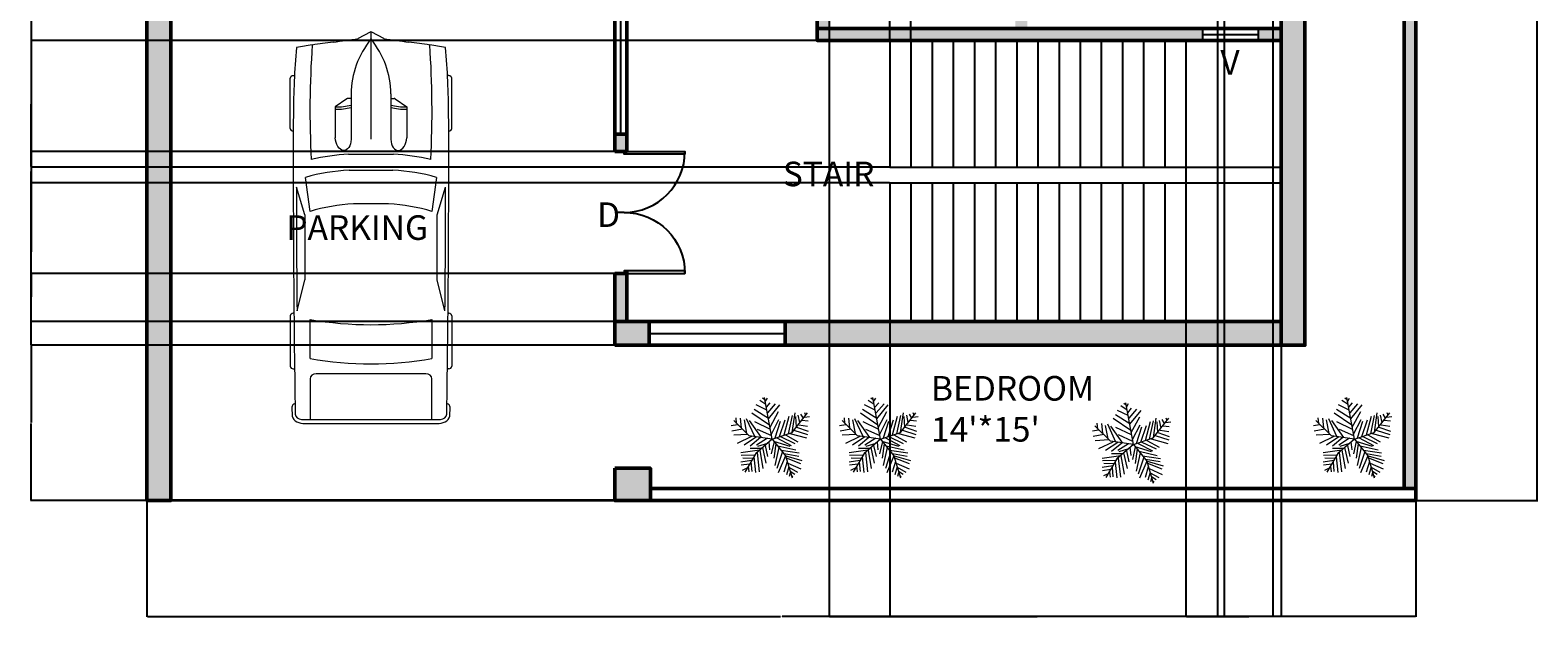
# Model space of a CAD drawing. Units: inches. Extents: x 2024 to 2594, y 643 to 1604.
# Tile 1 of 4: x 2024 to 2594, y 643 to 865. Entities that reach past the tile are written whole.
import ezdxf

# ---------------------------------------------------------------- set-up
doc = ezdxf.new("R2010")
doc.units = ezdxf.units.IN
for name, color, linetype, lineweight in [('A-ANNO-DIMS', 2, 'Continuous', 18), ('A-ANNO-TEXT', 7, 'Continuous', 18), ('A-AREA-IDEN', 7, 'Continuous', 25), ('A-FLOR-STRS', 7, 'Continuous', 25), ('A-WALL-PATT', 50, 'Continuous', 13), ('C-PRKG-VEHI', 8, 'Continuous', 18), ('C-PROP', 7, 'Continuous', 35), ('DOOR', 240, 'Continuous', 25), ('TREE', 102, 'Continuous', 18), ('WALL', 50, 'Continuous', 50), ('WIN', 140, 'Continuous', 25)]:
    doc.layers.add(name, color=color, linetype=linetype, lineweight=lineweight)
doc.styles.get("Standard").update_dxf_attribs({"font": 'arial.ttf'})
doc.dimstyles.get("Standard").update_dxf_attribs({"dimtxt": 0.18, "dimasz": 0.18, "dimexe": 0.18, "dimexo": 0.0625, "dimgap": 0.09, "dimtad": 0, "dimtih": 1, "dimtoh": 1, "dimdec": 4, "dimzin": 0, "dimdsep": 46, "dimtxsty": 'Standard', "dimcen": 0.09, "dimadec": 0, "dimazin": 0, "dimtfac": 1, "dimtdec": 4, "dimtofl": 0, "dimtmove": 0, "dimatfit": 3, "dimfxl": 1, "dimtolj": 1, "dimtzin": 0, "dimarcsym": 0})

# ---------------------------------------------------------------- blocks, each defined once
blk = doc.blocks.new('*U8')
for p, q in [((21.1, 37.41), (21.1, 36.83)), ((46.55, 38.89), (22.35, 38.89)), ((47.8, 37.39), (47.8, 37.41)), ((135.45, 37.07), (135.45, 37.41)), ((136.7, 38.89), (160.9, 38.89)), ((162.15, 37.41), (162.15, 36.77)), ((70.03, 31.54), (86.41, 29.35)), ((87.99, 31.87), (74.76, 35.92)), ((134.31, 35.6), (119.29, 31.78)), ((138.42, 29.35), (157.25, 29.35)), ((186.47, 29.35), (167.01, 29.35)), ((186.47, -33.5), (186.47, 33.5)), ((188.4, -32.76), (188.4, 32.76)), ((164.52, 26.39), (164.52, -26.39)), ((32.27, 11.63), (36.13, 17.17)), ((36.13, 17.17), (50.94, 17.17)), ((29.77, 9.51), (51.68, 9.51)), ((32.12, 9.51), (32.12, 11.15)), ((58.92, -10.77), (58.92, 10.77)), ((66.55, -10.53), (66.55, 10.53)), ((82.74, 8.5), (82.74, -8.5)), ((186.47, -10.53), (186.47, 10.53)), ((3.27, 6.13), (0.1, 0.41)), ((0, 0), (51.68, 0)), ((0.1, -0.41), (3.27, -6.13)), ((29.77, -9.51), (51.68, -9.51)), ((32.12, -9.51), (32.12, -11.15)), ((32.27, -11.63), (36.13, -17.17)), ((36.13, -17.17), (50.94, -17.17)), ((86.41, -29.35), (70.03, -31.54)), ((87.99, -31.87), (74.76, -35.92)), ((134.31, -35.6), (119.29, -31.78)), ((157.25, -29.35), (138.42, -29.35)), ((167.01, -29.35), (186.47, -29.35)), ((21.1, -37.41), (21.1, -36.83)), ((46.55, -38.89), (22.35, -38.89)), ((47.8, -37.39), (47.8, -37.41)), ((135.45, -37.07), (135.45, -37.41)), ((136.7, -38.89), (160.9, -38.89)), ((162.15, -37.41), (162.15, -36.77))]:
    blk.add_line(p, q)
for centre, major_axis, ratio, start_param, end_param in [((41.19, -490.86), (0, 528.23), 0.842304, 0.00281, 0.075598), ((22.35, 37.41), (0, -1.48), 0.842304, 3.141593, 4.712389), ((64.48, -10555.62), (0, 10593.03), 0.842304, -0.013397, 0.002797), ((46.55, 37.41), (0, 1.48), 0.842304, -1.570796, 0), ((136.7, 37.41), (0, -1.48), 0.842304, 3.141593, 4.712389), ((160.9, 37.41), (0, 1.48), 0.842304, -1.570796, 0), ((180.63, 35.84), (0, 2.22), 0.842304, -0.013017, 1.249894), ((64.48, -10556.36), (0, 10595.31), 0.842304, -0.013397, -0.013017), ((183.98, 33.5), (0, -2.96), 0.842304, 1.570796, 3.128196), ((183.98, 32.76), (0, -5.25), 0.842304, 1.570796, 3.128196), ((266.03, -27.52), (0, 313.31), 0.842304, 1.367076, 1.39176), ((37.47, -593.96), (0, -623.33), 0.842304, 3.096046, 3.200911), ((135.29, 5.39), (0, 81.77), 0.842304, 1.245306, 1.50788), ((64.48, -10555.62), (0, -10591.55), 0.842304, 3.133765, 3.140441), ((149.6, 2.8), (0, -79.58), 0.842304, 4.372215, 4.640744), ((95.79, -3666.35), (0, -3698.24), 0.842304, 3.134049, 3.144098), ((17.08, 0), (0, 147.02), 0.842304, 4.511394, 4.913384), ((35.91, 0), (0, 147.02), 0.842304, 4.511394, 4.913384), ((167.01, 26.39), (0, 2.96), 0.842304, 0, 1.570796), ((259.18, -27.52), (0, -305.3), 0.842304, 4.528606, 4.561838), ((134.4, 5.39), (0, -89.78), 0.842304, 4.449482, 4.652344), ((-204.49, 52.4), (0, -250.96), 0.842304, 1.385369, 1.434372), ((13.04, 17.01), (0, 27.42), 0.842304, 4.435146, 4.718221), ((14.2, 17.01), (0, 27.42), 0.842304, 4.435146, 4.718221), ((50.79, 13.34), (6.34, -0.36), 0.603834, -1.395552, 1.581315), ((29.77, -46.66), (0, 56.17), 0.842304, 0, 0.590319), ((32.75, 11.15), (0, 0.74), 0.842304, 0.879714, 1.570796), ((0.62, 0), (0, -0.74), 0.842304, 4.131459, 5.293319), ((-204.49, -52.4), (0, 250.96), 0.842304, -1.434372, -1.385369), ((29.77, 46.66), (0, 56.17), 0.842304, 2.551274, 3.141593), ((32.75, -11.15), (0, -0.74), 0.842304, 4.712389, 5.403472), ((13.04, -17.01), (0, -27.42), 0.842304, 1.564964, 1.848039), ((14.2, -17.01), (0, -27.42), 0.842304, 1.564964, 1.848039), ((134.4, -5.39), (0, -89.78), 0.842304, -1.510751, -1.307889), ((135.29, -5.39), (0, -81.77), 0.842304, -1.50788, -1.245306), ((149.6, -2.8), (0, -79.58), 0.842304, -1.499151, -1.230623), ((259.18, 27.52), (0, 305.3), 0.842304, 1.721348, 1.754579), ((266.03, 27.52), (0, 313.31), 0.842304, 1.749832, 1.774517), ((37.47, 593.96), (0, -623.33), 0.842304, -0.059319, 0.045547), ((167.01, -26.39), (0, -2.96), 0.842304, 4.712389, 6.283185), ((41.19, 490.86), (0, -528.23), 0.842304, -0.075598, -0.00281), ((64.48, 10555.62), (0, -10591.55), 0.842304, 0.001152, 0.007828), ((95.79, 3666.35), (0, -3698.24), 0.842304, -0.002505, 0.007544), ((183.98, -33.5), (0, 2.96), 0.842304, 3.15499, 4.712389), ((183.98, -32.76), (0, -5.25), 0.842304, 0.013397, 1.570796), ((22.35, -37.41), (0, 1.48), 0.842304, 1.570796, 3.141593), ((64.48, 10555.62), (0, 10593.03), 0.842304, 3.138796, 3.15499), ((46.55, -37.41), (0, -1.48), 0.842304, 0, 1.570796), ((136.7, -37.41), (0, -1.48), 0.842304, -1.570796, 0), ((160.9, -37.41), (0, 1.48), 0.842304, 3.141593, 4.712389), ((180.63, -35.84), (0, -2.22), 0.842304, -1.249894, 0.013017), ((64.48, 10556.36), (0, 10595.31), 0.842304, 3.15461, 3.15499)]:
    blk.add_ellipse(centre, major_axis=major_axis, ratio=ratio, start_param=start_param, end_param=end_param)
at = {"extrusion": (0, 0, -1)}
blk.add_ellipse((50.79, -13.34), major_axis=(6.34, 0.36), ratio=0.603834, start_param=-1.395552, end_param=1.581315, dxfattribs=at)
blk = doc.blocks.new('*U2')
for p, q in [((0, 0), (0, -6)), ((40, 0), (40, -6))]:
    blk.add_line(p, q)
blk.add_lwpolyline([(0, 0), (0, 40), (1.75, 40), (1.75, 0)], close=True)
blk.add_arc((0, 0), 40, 0, 90)
blk = doc.blocks.new('*U6')
for p, q in [((-7.288, 39.707), (-21.778, 46.673)), ((-8.737, 47.138), (-17.069, 52.711)), ((-10.186, 53.64), (-13.084, 55.962)), ((0, 0), (-10.5, 57)), ((-9.099, 51.782), (-6.563, 55.962)), ((-7.65, 43.423), (-2.578, 49.46)), ((-5.839, 35.992), (4.667, 48.067)), ((-5.114, 27.632), (10.463, 46.673)), ((-31.5, 4.5), (-52.5, 25.5)), ((-48.585, 21.131), (-49.309, 29.026)), ((-43.513, 28.561), (-42.427, 15.558)), ((-38.442, 26.239), (-34.819, 7.663)), ((-35.544, 28.097), (-24.314, 3.947)), ((-14.533, 2.09), (-30.834, 25.31)), ((-3.665, 19.273), (-27.574, 35.527)), ((-5.114, 28.097), (-24.676, 40.636)), ((-24.314, 23.917), (-2.941, 13.7)), ((-2.941, 16.486), (8.652, 37.85)), ((-1.129, 6.734), (9.014, 26.704)), ((3.942, 1.625), (11.187, 24.381)), ((10.101, 3.483), (17.708, 26.239)), ((16.259, 5.805), (23.142, 31.348)), ((22.055, 7.198), (27.489, 32.277)), ((27, 9), (48, 36)), ((27.127, 9.056), (31.112, 35.992)), ((31.836, 30.883), (32.561, 16.486)), ((35.096, 32.741), (37.27, 22.524)), ((38.719, 34.134), (41.979, 28.561)), ((40.53, 25.775), (48.862, 24.846)), ((43.791, 29.954), (51.036, 30.883)), ((44.153, 36.456), (45.239, 32.741)), ((-47.498, 19.737), (-55.83, 18.344)), ((-40.615, 13.7), (-55.105, 10.913)), ((-33.37, 6.269), (-52.207, 5.34)), ((-28.299, 3.483), (-47.86, -5.805)), ((-21.416, 3.018), (-38.079, -8.128)), ((0, 0), (-31.5, 4.5)), ((-15.982, 2.09), (-30.11, -9.521)), ((0, 0), (-22.5, -19.5)), ((-6.563, 1.161), (-21.416, -8.128)), ((-20.691, 13.7), (-1.129, 4.876)), ((0, 0), (27, 9)), ((0, 0), (18, -22.5)), ((6.478, 1.625), (26.04, -8.592)), ((11.187, 3.483), (30.749, -5.805)), ((18.07, 5.805), (35.096, -3.483)), ((24.229, 7.663), (46.688, 1.625)), ((29.662, 12.307), (48.137, 6.269)), ((33.285, 16.486), (48.862, 10.913)), ((36.183, 19.737), (48.137, 17.88)), ((-17.431, -15.094), (-42.789, -18.809)), ((-22.5, -19.5), (-37.5, -45)), ((-15.257, -12.772), (-30.11, -12.772)), ((-20.691, -18.345), (-17.793, -44.352)), ((-6.563, -5.805), (-19.967, -9.985)), ((-17.069, -15.094), (-12.721, -40.172)), ((-13.446, -11.378), (-8.737, -32.741)), ((-9.461, -8.592), (-6.201, -23.453)), ((-4.752, -3.483), (-3.665, -14.629)), ((2.493, -3.019), (-1.491, -20.202)), ((1.769, -2.555), (24.229, -9.521)), ((5.029, -6.27), (2.131, -25.775)), ((9.014, -11.378), (3.58, -35.992)), ((14.085, -16.951), (6.478, -40.172)), ((7.565, -9.056), (32.198, -14.629)), ((12.274, -15.094), (36.907, -18.809)), ((16.259, -19.738), (36.183, -22.989)), ((-28.299, -29.026), (-42.789, -31.348)), ((-24.314, -21.596), (-42.427, -22.06)), ((-30.834, -34.135), (-42.427, -35.528)), ((-34.457, -39.708), (-40.978, -42.494)), ((-26.849, -26.24), (-40.253, -25.775)), ((-32.646, -36.921), (-31.921, -44.352)), ((-29.023, -30.884), (-27.936, -43.887)), ((-25.038, -23.918), (-22.865, -45.281)), ((18.07, -22.524), (8.289, -45.745)), ((20.244, -30.419), (15.897, -44.816)), ((18, -22.5), (27, -52.5)), ((18.433, -22.524), (40.53, -29.026)), ((19.157, -25.311), (38.719, -33.206)), ((22.78, -37.85), (19.519, -48.532)), ((21.331, -32.741), (39.081, -40.636)), ((22.78, -38.314), (34.372, -44.816)), ((24.591, -45.745), (23.142, -50.854)), ((24.591, -43.423), (30.749, -47.603)), ((26.764, -49.925), (28.213, -50.854))]:
    blk.add_line(p, q)
blk = doc.blocks.new('*D25')
at = {"layer": 'A-ANNO-DIMS', "color": 0, "lineweight": -2, "transparency": 16777216}
for p, q in [((2068.27, 686.87), (2068.27, 642.95)), ((2548.27, 686.87), (2548.27, 642.95)), ((2068.45, 643.13), (2307.98, 643.13)), ((2548.09, 643.13), (2308.56, 643.13))]:
    blk.add_line(p, q, dxfattribs=at)
at = {"layer": 'A-ANNO-DIMS', "color": 0, "lineweight": 100, "transparency": 16777216}
for points in [[(2068.45, 643.16), (2068.45, 643.1), (2068.27, 643.13)], [(2548.09, 643.16), (2548.09, 643.1), (2548.27, 643.13)]]:
    blk.add_solid(points, dxfattribs=at)
at = {"layer": 'Defpoints', "color": 0, "lineweight": 100, "transparency": 16777216}
for p in [(2068.27, 686.93), (2548.27, 686.93), (2548.27, 643.13)]:
    blk.add_point(p, dxfattribs=at)
at = {"layer": 'A-ANNO-DIMS', "color": 0, "transparency": 16777216, "insert": (2308.27, 643.13), "char_height": 0.18, "attachment_point": 5}
blk.add_mtext('\\A1;480', dxfattribs=at)
blk = doc.blocks.new('*D26')
at = {"layer": 'A-ANNO-DIMS', "color": 0, "lineweight": -2, "transparency": 16777216}
for p, q in [((2548.34, 1526.93), (2594.37, 1526.93)), ((2594.19, 1526.75), (2594.19, 1107.11)), ((2594.19, 687.11), (2594.19, 1106.75)), ((2548.34, 686.93), (2594.37, 686.93))]:
    blk.add_line(p, q, dxfattribs=at)
at = {"layer": 'A-ANNO-DIMS', "color": 0, "lineweight": 100, "transparency": 16777216}
for points in [[(2594.16, 1526.75), (2594.22, 1526.75), (2594.19, 1526.93)], [(2594.16, 687.11), (2594.22, 687.11), (2594.19, 686.93)]]:
    blk.add_solid(points, dxfattribs=at)
at = {"layer": 'Defpoints', "color": 0, "lineweight": 100, "transparency": 16777216}
for p in [(2548.27, 1526.93), (2594.19, 1526.93), (2548.27, 686.93)]:
    blk.add_point(p, dxfattribs=at)
at = {"layer": 'A-ANNO-DIMS', "color": 0, "transparency": 16777216, "insert": (2594.19, 1106.93), "char_height": 0.18, "attachment_point": 5}
blk.add_mtext('\\A1;840', dxfattribs=at)
blk = doc.blocks.new('*D31')
at = {"layer": 'A-ANNO-DIMS', "color": 0, "lineweight": -2, "transparency": 16777216}
for p, q in [((2245.21, 745.67), (2024.29, 745.67)), ((2024.47, 745.49), (2024.47, 716.48)), ((2024.47, 687.11), (2024.47, 716.12)), ((2068.21, 686.93), (2024.29, 686.93))]:
    blk.add_line(p, q, dxfattribs=at)
at = {"layer": 'A-ANNO-DIMS', "color": 0, "lineweight": 100, "transparency": 16777216}
for points in [[(2024.44, 745.49), (2024.5, 745.49), (2024.47, 745.67)], [(2024.44, 687.11), (2024.5, 687.11), (2024.47, 686.93)]]:
    blk.add_solid(points, dxfattribs=at)
at = {"layer": 'Defpoints', "color": 0, "lineweight": 100, "transparency": 16777216}
for p in [(2024.47, 745.67), (2245.27, 745.67), (2068.27, 686.93)]:
    blk.add_point(p, dxfattribs=at)
at = {"layer": 'A-ANNO-DIMS', "color": 0, "transparency": 16777216, "insert": (2024.47, 716.3), "char_height": 0.18, "attachment_point": 5}
blk.add_mtext('\\A1;58.74', dxfattribs=at)
blk = doc.blocks.new('*D32')
at = {"layer": 'A-ANNO-DIMS', "color": 0, "lineweight": -2, "transparency": 16777216}
for p, q in [((2077.21, 877.43), (2024.29, 877.43)), ((2024.47, 877.25), (2024.47, 811.73)), ((2024.47, 745.85), (2024.47, 811.37)), ((2245.21, 745.67), (2024.29, 745.67))]:
    blk.add_line(p, q, dxfattribs=at)
at = {"layer": 'A-ANNO-DIMS', "color": 0, "lineweight": 100, "transparency": 16777216}
for points in [[(2024.44, 877.25), (2024.5, 877.25), (2024.47, 877.43)], [(2024.44, 745.85), (2024.5, 745.85), (2024.47, 745.67)]]:
    blk.add_solid(points, dxfattribs=at)
at = {"layer": 'Defpoints', "color": 0, "lineweight": 100, "transparency": 16777216}
for p in [(2024.47, 877.43), (2077.27, 877.43), (2245.27, 745.67)]:
    blk.add_point(p, dxfattribs=at)
at = {"layer": 'A-ANNO-DIMS', "color": 0, "transparency": 16777216, "insert": (2024.47, 811.55), "char_height": 0.18, "attachment_point": 5}
blk.add_mtext('\\A1;131.76', dxfattribs=at)
blk = doc.blocks.new('*D40')
at = {"layer": 'A-ANNO-DIMS', "color": 0, "lineweight": -2, "transparency": 16777216}
for p, q in [((2326.27, 1114.37), (2326.27, 642.95)), ((2473.27, 1114.37), (2473.27, 642.95)), ((2326.45, 643.13), (2399.49, 643.13)), ((2473.09, 643.13), (2400.05, 643.13))]:
    blk.add_line(p, q, dxfattribs=at)
at = {"layer": 'A-ANNO-DIMS', "color": 0, "lineweight": 100, "transparency": 16777216}
for points in [[(2326.45, 643.16), (2326.45, 643.1), (2326.27, 643.13)], [(2473.09, 643.16), (2473.09, 643.1), (2473.27, 643.13)]]:
    blk.add_solid(points, dxfattribs=at)
at = {"layer": 'Defpoints', "color": 0, "lineweight": 100, "transparency": 16777216}
for p in [(2326.27, 1114.43), (2473.27, 1114.43), (2473.27, 643.13)]:
    blk.add_point(p, dxfattribs=at)
at = {"layer": 'A-ANNO-DIMS', "color": 0, "transparency": 16777216, "insert": (2399.77, 643.13), "char_height": 0.18, "attachment_point": 5}
blk.add_mtext('\\A1;147', dxfattribs=at)
blk = doc.blocks.new('*D41')
at = {"layer": 'A-ANNO-DIMS', "color": 0, "lineweight": -2, "transparency": 16777216}
for p, q in [((2473.27, 1114.37), (2473.27, 642.95)), ((2497.27, 1090.37), (2497.27, 642.95)), ((2473.45, 643.13), (2485.05, 643.13)), ((2497.09, 643.13), (2485.49, 643.13))]:
    blk.add_line(p, q, dxfattribs=at)
at = {"layer": 'A-ANNO-DIMS', "color": 0, "lineweight": 100, "transparency": 16777216}
for points in [[(2473.45, 643.16), (2473.45, 643.1), (2473.27, 643.13)], [(2497.09, 643.16), (2497.09, 643.1), (2497.27, 643.13)]]:
    blk.add_solid(points, dxfattribs=at)
at = {"layer": 'Defpoints', "color": 0, "lineweight": 100, "transparency": 16777216}
for p in [(2473.27, 1114.43), (2497.27, 1090.43), (2497.27, 643.13)]:
    blk.add_point(p, dxfattribs=at)
at = {"layer": 'A-ANNO-DIMS', "color": 0, "transparency": 16777216, "insert": (2485.27, 643.13), "char_height": 0.18, "attachment_point": 5}
blk.add_mtext('\\A1;24', dxfattribs=at)
blk = doc.blocks.new('*D47')
at = {"layer": 'A-ANNO-DIMS', "color": 0, "lineweight": -2, "transparency": 16777216}
for p, q in [((2475.68, 1134.57), (2475.68, 642.95)), ((2494.15, 1134.57), (2494.15, 642.95)), ((2475.86, 643.13), (2484.53, 643.13)), ((2493.97, 643.13), (2485.3, 643.13))]:
    blk.add_line(p, q, dxfattribs=at)
at = {"layer": 'A-ANNO-DIMS', "color": 0, "lineweight": 100, "transparency": 16777216}
for points in [[(2475.86, 643.16), (2475.86, 643.1), (2475.68, 643.13)], [(2493.97, 643.16), (2493.97, 643.1), (2494.15, 643.13)]]:
    blk.add_solid(points, dxfattribs=at)
at = {"layer": 'Defpoints', "color": 0, "lineweight": 100, "transparency": 16777216}
for p in [(2475.68, 1134.64), (2494.15, 1134.64), (2494.15, 643.13)]:
    blk.add_point(p, dxfattribs=at)
at = {"layer": 'A-ANNO-DIMS', "color": 0, "transparency": 16777216, "insert": (2484.91, 643.13), "char_height": 0.18, "attachment_point": 5}
blk.add_mtext('\\A1;18.47', dxfattribs=at)
blk = doc.blocks.new('*D48')
at = {"layer": 'A-ANNO-DIMS', "color": 0, "lineweight": -2, "transparency": 16777216}
for p, q in [((2249.77, 819.02), (2249.77, 1603.82)), ((2249.95, 1603.64), (2299.2, 1603.64)), ((2349.09, 1603.64), (2299.85, 1603.64)), ((2349.27, 860.99), (2349.27, 1603.82))]:
    blk.add_line(p, q, dxfattribs=at)
at = {"layer": 'A-ANNO-DIMS', "color": 0, "lineweight": 100, "transparency": 16777216}
for points in [[(2249.95, 1603.67), (2249.95, 1603.61), (2249.77, 1603.64)], [(2349.09, 1603.67), (2349.09, 1603.61), (2349.27, 1603.64)]]:
    blk.add_solid(points, dxfattribs=at)
at = {"layer": 'Defpoints', "color": 0, "lineweight": 100, "transparency": 16777216}
for p in [(2349.27, 1603.64), (2349.27, 860.93), (2249.77, 818.96)]:
    blk.add_point(p, dxfattribs=at)
at = {"layer": 'A-ANNO-DIMS', "color": 0, "transparency": 16777216, "insert": (2299.52, 1603.64), "char_height": 0.18, "attachment_point": 5}
blk.add_mtext('\\A1;99.5', dxfattribs=at)
blk = doc.blocks.new('*D49')
at = {"layer": 'A-ANNO-DIMS', "color": 0, "lineweight": -2, "transparency": 16777216}
for p, q in [((2349.27, 754.6), (2349.27, 642.95)), ((2461.27, 754.6), (2461.27, 642.95)), ((2349.45, 643.13), (2404.99, 643.13)), ((2461.09, 643.13), (2405.55, 643.13))]:
    blk.add_line(p, q, dxfattribs=at)
at = {"layer": 'A-ANNO-DIMS', "color": 0, "lineweight": 100, "transparency": 16777216}
for points in [[(2349.45, 643.16), (2349.45, 643.1), (2349.27, 643.13)], [(2461.09, 643.16), (2461.09, 643.1), (2461.27, 643.13)]]:
    blk.add_solid(points, dxfattribs=at)
at = {"layer": 'Defpoints', "color": 0, "lineweight": 100, "transparency": 16777216}
for p in [(2349.27, 754.67), (2461.27, 754.67), (2461.27, 643.13)]:
    blk.add_point(p, dxfattribs=at)
at = {"layer": 'A-ANNO-DIMS', "color": 0, "transparency": 16777216, "insert": (2405.27, 643.13), "char_height": 0.18, "attachment_point": 5}
blk.add_mtext('\\A1;112', dxfattribs=at)
blk = doc.blocks.new('*D50')
at = {"layer": 'A-ANNO-DIMS', "color": 0, "lineweight": -2, "transparency": 16777216}
for p, q in [((2461.27, 754.6), (2461.27, 642.95)), ((2497.27, 754.6), (2497.27, 642.95)), ((2461.45, 643.13), (2479.05, 643.13)), ((2497.09, 643.13), (2479.49, 643.13))]:
    blk.add_line(p, q, dxfattribs=at)
at = {"layer": 'A-ANNO-DIMS', "color": 0, "lineweight": 100, "transparency": 16777216}
for points in [[(2461.45, 643.16), (2461.45, 643.1), (2461.27, 643.13)], [(2497.09, 643.16), (2497.09, 643.1), (2497.27, 643.13)]]:
    blk.add_solid(points, dxfattribs=at)
at = {"layer": 'Defpoints', "color": 0, "lineweight": 100, "transparency": 16777216}
for p in [(2461.27, 754.67), (2497.27, 754.67), (2497.27, 643.13)]:
    blk.add_point(p, dxfattribs=at)
at = {"layer": 'A-ANNO-DIMS', "color": 0, "transparency": 16777216, "insert": (2479.27, 643.13), "char_height": 0.18, "attachment_point": 5}
blk.add_mtext('\\A1;36', dxfattribs=at)
blk = doc.blocks.new('*D51')
at = {"layer": 'A-ANNO-DIMS', "color": 0, "lineweight": -2, "transparency": 16777216}
for p, q in [((2349.27, 860.99), (2349.27, 1603.82)), ((2349.45, 1603.64), (2353.12, 1603.64)), ((2357.09, 1603.64), (2353.42, 1603.64)), ((2357.27, 860.99), (2357.27, 1603.82))]:
    blk.add_line(p, q, dxfattribs=at)
at = {"layer": 'A-ANNO-DIMS', "color": 0, "lineweight": 100, "transparency": 16777216}
for points in [[(2349.45, 1603.67), (2349.45, 1603.61), (2349.27, 1603.64)], [(2357.09, 1603.67), (2357.09, 1603.61), (2357.27, 1603.64)]]:
    blk.add_solid(points, dxfattribs=at)
at = {"layer": 'Defpoints', "color": 0, "lineweight": 100, "transparency": 16777216}
for p in [(2357.27, 1603.64), (2349.27, 860.93), (2357.27, 860.93)]:
    blk.add_point(p, dxfattribs=at)
at = {"layer": 'A-ANNO-DIMS', "color": 0, "transparency": 16777216, "insert": (2353.27, 1603.64), "char_height": 0.18, "attachment_point": 5}
blk.add_mtext('\\A1;8', dxfattribs=at)
blk = doc.blocks.new('*D52')
at = {"layer": 'A-ANNO-DIMS', "color": 0, "lineweight": -2, "transparency": 16777216}
for p, q in [((2349.21, 807.05), (2024.29, 807.05)), ((2024.47, 806.87), (2024.47, 781.04)), ((2024.47, 754.85), (2024.47, 780.68)), ((2349.21, 754.67), (2024.29, 754.67))]:
    blk.add_line(p, q, dxfattribs=at)
at = {"layer": 'A-ANNO-DIMS', "color": 0, "lineweight": 100, "transparency": 16777216}
for points in [[(2024.44, 806.87), (2024.5, 806.87), (2024.47, 807.05)], [(2024.44, 754.85), (2024.5, 754.85), (2024.47, 754.67)]]:
    blk.add_solid(points, dxfattribs=at)
at = {"layer": 'Defpoints', "color": 0, "lineweight": 100, "transparency": 16777216}
for p in [(2024.47, 807.05), (2349.27, 807.05), (2349.27, 754.67)]:
    blk.add_point(p, dxfattribs=at)
at = {"layer": 'A-ANNO-DIMS', "color": 0, "transparency": 16777216, "insert": (2024.47, 780.86), "char_height": 0.18, "attachment_point": 5}
blk.add_mtext('\\A1;52.38', dxfattribs=at)
blk = doc.blocks.new('*D53')
at = {"layer": 'A-ANNO-DIMS', "color": 0, "lineweight": -2, "transparency": 16777216}
for p, q in [((2349.21, 813.05), (2024.29, 813.05)), ((2024.47, 812.87), (2024.47, 810.23)), ((2024.47, 807.23), (2024.47, 809.87)), ((2349.21, 807.05), (2024.29, 807.05))]:
    blk.add_line(p, q, dxfattribs=at)
at = {"layer": 'A-ANNO-DIMS', "color": 0, "lineweight": 100, "transparency": 16777216}
for points in [[(2024.44, 812.87), (2024.5, 812.87), (2024.47, 813.05)], [(2024.44, 807.23), (2024.5, 807.23), (2024.47, 807.05)]]:
    blk.add_solid(points, dxfattribs=at)
at = {"layer": 'Defpoints', "color": 0, "lineweight": 100, "transparency": 16777216}
for p in [(2024.47, 813.05), (2349.27, 813.05), (2349.27, 807.05)]:
    blk.add_point(p, dxfattribs=at)
at = {"layer": 'A-ANNO-DIMS', "color": 0, "transparency": 16777216, "insert": (2024.47, 810.05), "char_height": 0.18, "attachment_point": 5}
blk.add_mtext('\\A1;6', dxfattribs=at)
blk = doc.blocks.new('*D54')
at = {"layer": 'A-ANNO-DIMS', "color": 0, "lineweight": -2, "transparency": 16777216}
for p, q in [((2349.21, 860.93), (2024.29, 860.93)), ((2024.47, 860.75), (2024.47, 837.17)), ((2024.47, 813.23), (2024.47, 836.81)), ((2349.21, 813.05), (2024.29, 813.05))]:
    blk.add_line(p, q, dxfattribs=at)
at = {"layer": 'A-ANNO-DIMS', "color": 0, "lineweight": 100, "transparency": 16777216}
for points in [[(2024.44, 860.75), (2024.5, 860.75), (2024.47, 860.93)], [(2024.44, 813.23), (2024.5, 813.23), (2024.47, 813.05)]]:
    blk.add_solid(points, dxfattribs=at)
at = {"layer": 'Defpoints', "color": 0, "lineweight": 100, "transparency": 16777216}
for p in [(2024.47, 860.93), (2349.27, 860.93), (2349.27, 813.05)]:
    blk.add_point(p, dxfattribs=at)
at = {"layer": 'A-ANNO-DIMS', "color": 0, "transparency": 16777216, "insert": (2024.47, 836.99), "char_height": 0.18, "attachment_point": 5}
blk.add_mtext('\\A1;47.88', dxfattribs=at)
blk = doc.blocks.new('*D55')
at = {"layer": 'A-ANNO-DIMS', "color": 0, "lineweight": -2, "transparency": 16777216}
for p, q in [((2245.21, 772.85), (2024.29, 772.85)), ((2024.47, 772.67), (2024.47, 763.94)), ((2024.47, 754.85), (2024.47, 763.58)), ((2249.71, 754.67), (2024.29, 754.67))]:
    blk.add_line(p, q, dxfattribs=at)
at = {"layer": 'A-ANNO-DIMS', "color": 0, "lineweight": 100, "transparency": 16777216}
for points in [[(2024.44, 772.67), (2024.5, 772.67), (2024.47, 772.85)], [(2024.44, 754.85), (2024.5, 754.85), (2024.47, 754.67)]]:
    blk.add_solid(points, dxfattribs=at)
at = {"layer": 'Defpoints', "color": 0, "lineweight": 100, "transparency": 16777216}
for p in [(2024.47, 772.85), (2245.27, 772.85), (2249.77, 754.67)]:
    blk.add_point(p, dxfattribs=at)
at = {"layer": 'A-ANNO-DIMS', "color": 0, "transparency": 16777216, "insert": (2024.47, 763.76), "char_height": 0.18, "attachment_point": 5}
blk.add_mtext('\\A1;18.187', dxfattribs=at)
blk = doc.blocks.new('*D56')
at = {"layer": 'A-ANNO-DIMS', "color": 0, "lineweight": -2, "transparency": 16777216}
for p, q in [((2245.21, 818.96), (2024.29, 818.96)), ((2024.47, 818.78), (2024.47, 796.09)), ((2024.47, 773.03), (2024.47, 795.72)), ((2245.21, 772.85), (2024.29, 772.85))]:
    blk.add_line(p, q, dxfattribs=at)
at = {"layer": 'A-ANNO-DIMS', "color": 0, "lineweight": 100, "transparency": 16777216}
for points in [[(2024.44, 818.78), (2024.5, 818.78), (2024.47, 818.96)], [(2024.44, 773.03), (2024.5, 773.03), (2024.47, 772.85)]]:
    blk.add_solid(points, dxfattribs=at)
at = {"layer": 'Defpoints', "color": 0, "lineweight": 100, "transparency": 16777216}
for p in [(2024.47, 818.96), (2245.27, 818.96), (2245.27, 772.85)]:
    blk.add_point(p, dxfattribs=at)
at = {"layer": 'A-ANNO-DIMS', "color": 0, "transparency": 16777216, "insert": (2024.47, 795.9), "char_height": 0.18, "attachment_point": 5}
blk.add_mtext('\\A1;46.1', dxfattribs=at)

msp = doc.modelspace()

# ---------------------------------------------------------------- hatches: boundary and pattern name
at = {"layer": 'A-WALL-PATT'}
h = msp.add_hatch(color=256, dxfattribs=at)
h.dxf.hatch_style = 1
h.paths.add_polyline_path([(2543.7727, 1526.9303), (2077.2727, 1526.9303), (2077.2727, 1522.4303), (2543.7727, 1522.4303)])
h.paths.add_polyline_path([(2077.2727, 1526.9303), (2068.2727, 1526.9303), (2068.2727, 1475.9303), (2077.2727, 1475.9303)])
h.paths.add_polyline_path([(2077.2727, 1475.9303), (2068.2727, 1475.9303), (2068.2727, 686.9303), (2077.2727, 686.9303)])
h.paths.add_polyline_path([(2548.2727, 1526.9303), (2543.7727, 1526.9303), (2543.7727, 1522.4303), (2543.7727, 691.4303), (2548.2727, 691.4303)])
h.paths.add_polyline_path([(2249.7727, 1078.4303), (2199.5227, 1078.4303), (2199.5227, 1073.9303), (2245.2727, 1073.9303), (2249.7727, 1073.9217)])
h.paths.add_polyline_path([(2249.7727, 1073.9217), (2245.2727, 1073.9217), (2245.2727, 935.5102), (2249.7727, 935.5102)])
h.paths.add_polyline_path([(2326.2727, 1121.201), (2321.7727, 1121.201), (2321.7727, 1085.9303), (2326.2727, 1085.9303), (2326.2727, 1090.4303)])
h.paths.add_polyline_path([(2497.2727, 1090.4303), (2326.2727, 1090.4303), (2326.2727, 1085.9303), (2497.2727, 1085.9303)])
h.paths.add_polyline_path([(2326.2727, 1085.9303), (2321.7727, 1085.9303), (2321.7727, 989.0099), (2326.2727, 989.0099)])
h.paths.add_polyline_path([(2199.1605, 1286.9303), (2077.2727, 1286.9303), (2077.2727, 1282.4303), (2199.1605, 1282.4303)])
h.paths.add_polyline_path([(2321.7727, 1286.9303), (2239.1605, 1286.9303), (2239.1605, 1282.4303), (2321.7727, 1282.4303)])
h.paths.add_polyline_path([(2245.2727, 881.9303), (2214.9534, 881.9303), (2214.9534, 877.4303), (2245.2727, 877.4303)])
h.paths.add_polyline_path([(2118.9166, 881.9303), (2077.2727, 881.9303), (2077.2727, 877.4303), (2118.9166, 877.4303)])
h.paths.add_polyline_path([(2249.7727, 889.4074), (2246.315, 889.4074), (2245.2727, 889.4074), (2245.2727, 872.2078), (2249.7727, 872.2078)])
h.paths.add_polyline_path([(2405.0472, 941.9303), (2326.2727, 941.9303), (2326.2727, 937.4303), (2405.0472, 937.4303)])
h.paths.add_polyline_path([(2326.2727, 949.0099), (2321.7727, 949.0099), (2321.7727, 902.6727), (2326.2727, 902.6727)])
h.paths.add_polyline_path([(2326.2727, 871.366), (2321.7727, 871.366), (2321.7727, 865.4303), (2326.2727, 865.4303)])
h.paths.add_polyline_path([(2401.2727, 937.4303), (2396.7727, 937.4303), (2396.7727, 865.4303), (2401.2727, 865.4303)])
h.paths.add_polyline_path([(2497.2727, 941.9303), (2436.2168, 941.9303), (2436.2168, 937.4303), (2497.2727, 937.4303)])
h.paths.add_polyline_path([(2506.2727, 977.6959), (2497.2727, 977.6959), (2497.2727, 745.6665), (2506.2727, 745.6665)])
h.paths.add_polyline_path([(2497.2727, 754.6665), (2309.6667, 754.6665), (2309.6667, 745.6665), (2497.2727, 745.6665)])
h.paths.add_polyline_path([(2258.2092, 754.6665), (2245.2727, 754.6665), (2245.2727, 745.6665), (2258.2092, 745.6665)])
h.paths.add_polyline_path([(2249.7727, 772.853), (2248.7304, 772.853), (2245.2727, 772.853), (2245.2727, 754.6665), (2249.7727, 754.6665)])
h.paths.add_polyline_path([(2249.7727, 825.5234), (2245.2727, 825.5234), (2245.2727, 818.9558), (2248.7304, 818.9558), (2249.7727, 818.9558)])
h.paths.add_polyline_path([(2105.513, 1078.4303), (2077.2727, 1078.4303), (2077.2727, 1073.9303), (2105.513, 1073.9303)])
h.paths.add_polyline_path([(2326.2727, 1466.9303), (2321.7727, 1466.9303), (2321.7727, 1267.3126), (2326.2727, 1267.3126)])
h.paths.add_polyline_path([(2405.7727, 1466.9303), (2401.2727, 1466.9303), (2401.2727, 1438.953), (2405.7727, 1438.953)])
h.paths.add_polyline_path([(2405.7727, 1398.953), (2401.2727, 1398.953), (2401.2727, 1394.9303), (2405.7727, 1394.9303)])
h.paths.add_polyline_path([(2467.5339, 860.9303), (2467.5339, 865.4303), (2321.7727, 865.4303), (2321.7727, 860.9303)])
h.paths.add_polyline_path([(2488.7331, 865.4303), (2488.7331, 860.9303), (2497.2727, 860.9303), (2497.2727, 865.4303)])
h = msp.add_hatch(color=256, dxfattribs=at)
h.dxf.hatch_style = 1
h.paths.add_polyline_path([(2258.7401, 699.1454), (2245.2727, 699.1454), (2245.2727, 686.9303), (2258.7401, 686.9303), (2258.7401, 691.4303)])

# ---------------------------------------------------------------- linework, layer by layer
at = {"layer": 'A-FLOR-STRS'}
for p, q in [((2349.2727, 860.9303), (2349.2727, 813.0484)), ((2357.2727, 860.9303), (2357.2727, 813.0484)), ((2365.2727, 860.9303), (2365.2727, 813.0484)), ((2373.2727, 860.9303), (2373.2727, 813.0484)), ((2381.2727, 860.9303), (2381.2727, 813.0484)), ((2389.2727, 860.9303), (2389.2727, 813.0484)), ((2397.2727, 860.9303), (2397.2727, 813.0484)), ((2405.2727, 860.9303), (2405.2727, 813.0484)), ((2413.2727, 860.9303), (2413.2727, 813.0484)), ((2421.2727, 860.9303), (2421.2727, 813.0484)), ((2429.2727, 860.9303), (2429.2727, 813.0484)), ((2437.2727, 860.9303), (2437.2727, 813.0484)), ((2445.2727, 860.9303), (2445.2727, 813.0484)), ((2453.2727, 860.9303), (2453.2727, 813.0484)), ((2497.2727, 860.9303), (2461.2727, 860.9303)), ((2461.2727, 860.9303), (2461.2727, 754.6665)), ((2349.2727, 813.0484), (2497.2727, 813.0484)), ((2349.2727, 807.0484), (2497.2727, 807.0484)), ((2349.2727, 807.0484), (2349.2727, 754.6665)), ((2357.2727, 807.0484), (2357.2727, 754.6665)), ((2365.2727, 807.0484), (2365.2727, 754.6665)), ((2373.2727, 807.0484), (2373.2727, 754.6665)), ((2381.2727, 807.0484), (2381.2727, 754.6665)), ((2389.2727, 807.0484), (2389.2727, 754.6665)), ((2397.2727, 807.0484), (2397.2727, 754.6665)), ((2405.2727, 807.0484), (2405.2727, 754.6665)), ((2413.2727, 807.0484), (2413.2727, 754.6665)), ((2421.2727, 807.0484), (2421.2727, 754.6665)), ((2429.2727, 807.0484), (2429.2727, 754.6665)), ((2437.2727, 807.0484), (2437.2727, 754.6665)), ((2445.2727, 807.0484), (2445.2727, 754.6665)), ((2453.2727, 807.0484), (2453.2727, 754.6665))]:
    msp.add_line(p, q, dxfattribs=at)
at = {"layer": 'C-PROP'}
for p, q in [((2068.2727, 686.9303), (2068.2727, 1526.9303)), ((2548.2727, 1526.9303), (2548.2727, 686.9303)), ((2548.2727, 686.9303), (2068.2727, 686.9303))]:
    msp.add_line(p, q, dxfattribs=at)
msp.add_lwpolyline([(2548.2727, 686.9303), (2068.2727, 686.9303), (2068.2727, 1526.9303), (2548.2727, 1526.9303)], close=True, dxfattribs=at)
at = {"layer": 'WALL'}
for p, q in [((2506.2727, 1475.9303), (2506.2727, 745.6665)), ((2497.2727, 1466.9303), (2497.2727, 754.6665)), ((2245.2727, 877.4303), (2245.2727, 818.9558)), ((2249.7727, 877.4303), (2249.7727, 818.9558)), ((2321.7727, 860.9303), (2321.7727, 871.366)), ((2497.2727, 860.9303), (2321.7727, 860.9303)), ((2249.7727, 795.928), (2249.7727, 795.8809)), ((2245.2727, 772.853), (2245.2727, 745.6665)), ((2249.7727, 773.8615), (2249.7727, 754.6665)), ((2497.2727, 754.6665), (2249.7727, 754.6665)), ((2506.2727, 745.6665), (2245.2727, 745.6665)), ((2077.2727, 695.9303), (2077.2727, 686.9303)), ((2497.2727, 695.9303), (2497.2727, 695.9303))]:
    msp.add_line(p, q, dxfattribs=at)
for points in [[(2543.7727, 691.4303), (2548.2727, 691.4303), (2548.2727, 1526.9303), (2543.7727, 1526.9303)], [(2068.2727, 1475.9303), (2077.2727, 1475.9303), (2077.2727, 686.9303), (2068.2727, 686.9303)], [(2497.2727, 977.6959), (2506.2727, 977.6959), (2506.2727, 745.6665), (2497.2727, 745.6665)], [(2321.7727, 865.4303), (2497.2727, 865.4303), (2497.2727, 860.9303), (2321.7727, 860.9303)], [(2245.2727, 818.9558), (2249.7727, 818.9558), (2249.7727, 825.5234), (2245.2727, 825.5234)], [(2245.2727, 772.853), (2249.7727, 772.853), (2249.7727, 754.6665), (2245.2727, 754.6665)], [(2245.2727, 745.6665), (2258.2092, 745.6665), (2258.2092, 754.6665), (2245.2727, 754.6665)], [(2497.2727, 754.6665), (2309.6667, 754.6665), (2309.6667, 745.6665), (2497.2727, 745.6665)], [(2245.2727, 699.1454), (2258.7401, 699.1454), (2258.7401, 686.9303), (2245.2727, 686.9303)], [(2258.7401, 691.4303), (2548.2727, 691.4303), (2548.2727, 686.9303), (2258.7401, 686.9303)]]:
    msp.add_lwpolyline(points, close=True, dxfattribs=at)
for points in [[(2077.2727, 1522.4303), (2543.7727, 1522.4303), (2543.7727, 691.4303), (2258.7401, 691.4303)], [(2077.2727, 695.9303), (2077.2727, 877.4303)]]:
    msp.add_lwpolyline(points, dxfattribs=at)
at = {"layer": 'WIN'}
for p, q in [((2247.5227, 825.5234), (2247.5227, 872.2078)), ((2467.5339, 863.1803), (2488.7331, 863.1803)), ((2258.2092, 750.1665), (2309.6667, 750.1665))]:
    msp.add_line(p, q, dxfattribs=at)
for points in [[(2245.2727, 825.5234), (2249.7727, 825.5234), (2249.7727, 872.2078), (2245.2727, 872.2078)], [(2467.5339, 860.9303), (2488.7331, 860.9303), (2488.7331, 865.4303), (2467.5339, 865.4303)], [(2258.2092, 754.6665), (2309.6667, 754.6665), (2309.6667, 745.6665), (2258.2092, 745.6665)]]:
    msp.add_lwpolyline(points, close=True, dxfattribs=at)

# ---------------------------------------------------------------- block references
at = {"layer": 'C-PRKG-VEHI', "xscale": 0.7860108216162027, "yscale": 0.7860108216162027, "zscale": 0.7860108216162027, "rotation": 270}
msp.add_blockref('*U8', (2153.0247, 864.2093), dxfattribs=at)
at = {"layer": 'DOOR', "yscale": 0.5762850341581635, "zscale": 0.5762850341581635, "rotation": 270}
for p, xscale in [((2248.7304, 818.9558), 0.5762850341581635), ((2248.7304, 772.853), -0.5762850341581635)]:
    msp.add_blockref('*U2', p, dxfattribs=dict(at, xscale=xscale))
at = {"layer": 'TREE', "xscale": 0.2775790715638129, "yscale": 0.2775790715638129, "zscale": 0.2775790715638129}
for p in [(2304.7881, 710.1455), (2345.7832, 710.1455), (2525.0359, 710.1455), (2441.4382, 708.0927)]:
    msp.add_blockref('*U6', p, dxfattribs=at)

# ---------------------------------------------------------------- texts
at = {"layer": 'A-ANNO-TEXT', "char_height": 9.3008, "attachment_point": 1}
for s, insert in [('V', (2474.3059, 857.3487)), ('D', (2238.5221, 799.7014))]:
    msp.add_mtext_dynamic_manual_height_columns(s, width=384.915388, gutter_width=46.5039, heights=[0], dxfattribs=dict(at, insert=insert))
at = {"layer": 'A-AREA-IDEN', "char_height": 9.30079, "attachment_point": 1}
for s, insert in [('STAIR', (2308.7925, 815.1013)), ('PARKING', (2120.9956, 794.8133)), ("BEDROOM\\P14'*15'", (2364.8552, 734.0301))]:
    msp.add_mtext_dynamic_manual_height_columns(s, width=384.915388, gutter_width=46.5039, heights=[0], dxfattribs=dict(at, insert=insert))

# ---------------------------------------------------------------- dimensions: what is measured, and where the dimension line sits
at = {"layer": 'A-ANNO-DIMS'}
for base, p1, p2, override, picture, middle in [((2349.2727, 1603.6424), (2249.7727, 818.9558), (2349.2727, 860.9303), {"dimdec": 1, "dimlfac": 1, "dimrnd": 0, "dimzin": 0, "dimdsep": 46, "dimlunit": 2}, '*D48', (2299.5227, 1603.6424)), ((2357.2727, 1603.6424), (2349.2727, 860.9303), (2357.2727, 860.9303), {"dimdec": 0, "dimlfac": 1, "dimrnd": 0, "dimzin": 0, "dimdsep": 46, "dimlunit": 2}, '*D51', (2353.2727, 1603.6424)), ((2494.1482, 643.1303), (2475.6764, 1134.6374), (2494.1482, 1134.6374), {"dimdec": 2, "dimlfac": 1, "dimrnd": 0, "dimzin": 0, "dimdsep": 46, "dimlunit": 2}, '*D47', (2484.9123, 643.1303)), ((2473.2727, 643.1303), (2326.2727, 1114.4303), (2473.2727, 1114.4303), {"dimdec": 0, "dimlfac": 1, "dimrnd": 0, "dimzin": 0, "dimdsep": 46, "dimlunit": 2}, '*D40', (2399.7727, 643.1303)), ((2497.2727, 643.1303), (2473.2727, 1114.4303), (2497.2727, 1090.4303), {"dimdec": 0, "dimlfac": 1, "dimrnd": 0, "dimzin": 0, "dimdsep": 46, "dimlunit": 2}, '*D41', (2485.2727, 643.1303)), ((2461.2727, 643.1303), (2349.2727, 754.6665), (2461.2727, 754.6665), {"dimdec": 0, "dimlfac": 1, "dimrnd": 0, "dimzin": 0, "dimdsep": 46, "dimlunit": 2}, '*D49', (2405.2727, 643.1303)), ((2497.2727, 643.1303), (2461.2727, 754.6665), (2497.2727, 754.6665), {"dimdec": 0, "dimlfac": 1, "dimrnd": 0, "dimzin": 0, "dimdsep": 46, "dimlunit": 2}, '*D50', (2479.2727, 643.1303)), ((2548.2727, 643.1303), (2068.2727, 686.9303), (2548.2727, 686.9303), {"dimdec": 0, "dimlfac": 1, "dimrnd": 0, "dimzin": 0, "dimdsep": 46, "dimlunit": 2}, '*D25', (2308.2727, 643.1303))]:
    dim = msp.add_linear_dim(base=base, p1=p1, p2=p2, dimstyle='Standard', override=override, dxfattribs=at)
    dim.commit()
    dim.dimension.update_dxf_attribs({"geometry": picture, "text_midpoint": middle})
for base, p1, p2, override, picture, middle in [((2594.1903, 1526.9303), (2548.2727, 686.9303), (2548.2727, 1526.9303), {"dimdec": 0, "dimlfac": 1, "dimrnd": 0, "dimzin": 0, "dimdsep": 46, "dimlunit": 2}, '*D26', (2594.1903, 1106.9303)), ((2024.4727, 877.4303), (2245.2727, 745.6665), (2077.2727, 877.4303), {"dimdec": 2, "dimlfac": 1, "dimrnd": 0, "dimzin": 0, "dimdsep": 46, "dimlunit": 2}, '*D32', (2024.4727, 811.5484)), ((2024.4727, 860.9303), (2349.2727, 813.0484), (2349.2727, 860.9303), {"dimdec": 2, "dimlfac": 1, "dimrnd": 0, "dimzin": 0, "dimdsep": 46, "dimlunit": 2}, '*D54', (2024.4727, 836.9893)), ((2024.4727, 818.9558), (2245.2727, 772.853), (2245.2727, 818.9558), {"dimdec": 1, "dimlfac": 1, "dimrnd": 0, "dimzin": 0, "dimdsep": 46, "dimlunit": 2}, '*D56', (2024.4727, 795.9044)), ((2024.4727, 813.0484), (2349.2727, 807.0484), (2349.2727, 813.0484), {"dimdec": 0, "dimlfac": 1, "dimrnd": 0, "dimzin": 0, "dimdsep": 46, "dimlunit": 2}, '*D53', (2024.4727, 810.0484)), ((2024.4727, 807.0484), (2349.2727, 754.6665), (2349.2727, 807.0484), {"dimdec": 2, "dimlfac": 1, "dimrnd": 0, "dimzin": 0, "dimdsep": 46, "dimlunit": 2}, '*D52', (2024.4727, 780.8575)), ((2024.4727, 772.85304), (2249.7727, 754.66651), (2245.2727, 772.85304), {"dimdec": 3, "dimlfac": 1, "dimrnd": 0, "dimzin": 0, "dimdsep": 46, "dimlunit": 2}, '*D55', (2024.4727, 763.75978)), ((2024.4727, 745.6665), (2068.2727, 686.9303), (2245.2727, 745.6665), {"dimdec": 2, "dimlfac": 1, "dimrnd": 0, "dimzin": 0, "dimdsep": 46, "dimlunit": 2}, '*D31', (2024.4727, 716.2984))]:
    dim = msp.add_linear_dim(base=base, p1=p1, p2=p2, angle=90, dimstyle='Standard', override=override, dxfattribs=at)
    dim.commit()
    dim.dimension.update_dxf_attribs({"geometry": picture, "text_midpoint": middle})

doc.saveas('drawing.dxf')
